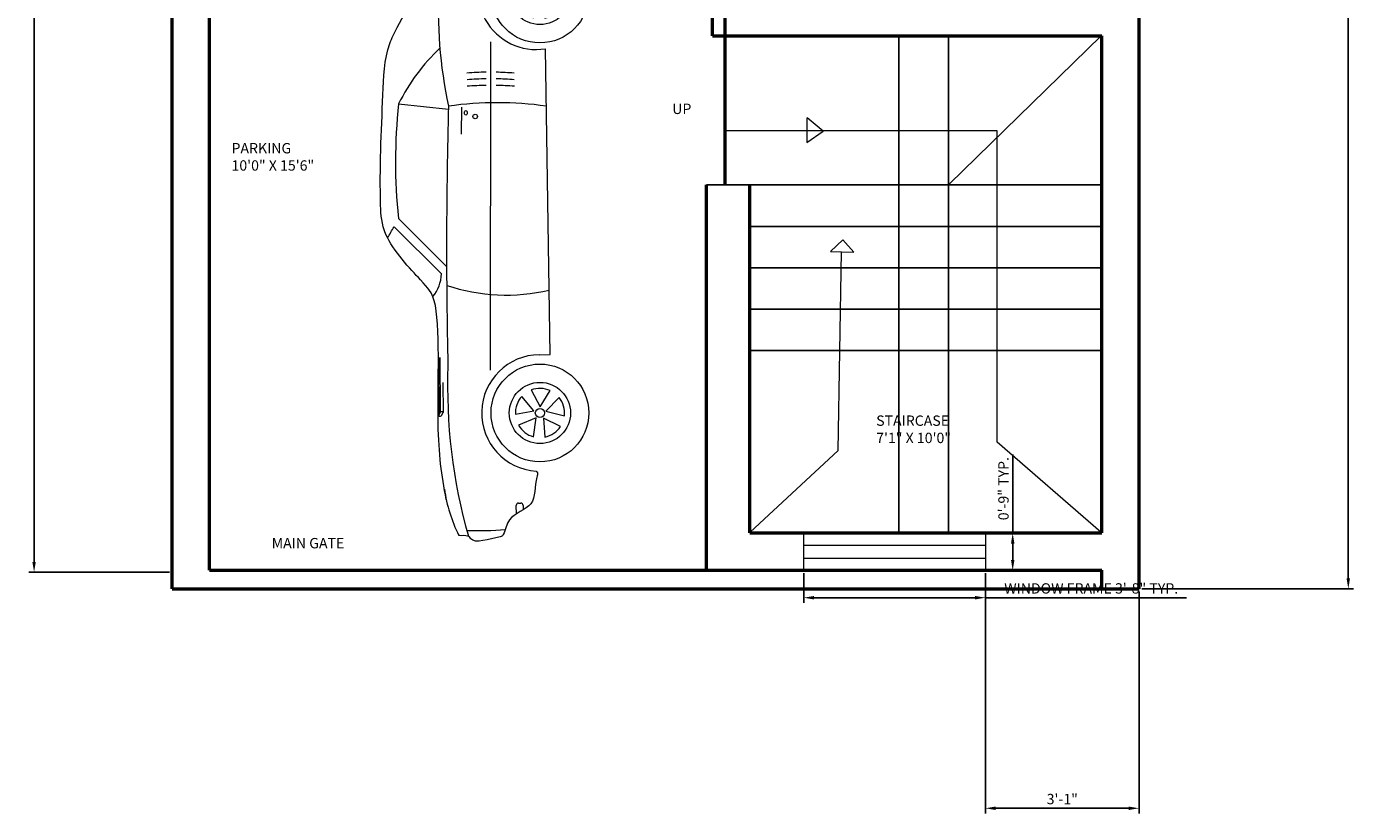
# Model space of a CAD drawing. Units: inches. Extents: x 210 to 950, y 0 to 561.
# Tile 1 of 5: x 228 to 548, y 0 to 190. Entities that reach past the tile are written whole.
import ezdxf

# ---------------------------------------------------------------- set-up
doc = ezdxf.new("R2010")
doc.units = ezdxf.units.IN
for name, color, linetype, lineweight in [('A-ANNO-DIMS', 2, 'Continuous', 18), ('A-ANNO-SYMB', 7, 'Continuous', 18), ('A-ANNO-TEXT', 7, 'Continuous', 18), ('A-AREA-IDEN', 7, 'Continuous', 18), ('A-FLOR-STRS', 7, 'Continuous', 25), ('A-GLAZ', 4, 'Continuous', 20), ('A-SITE-VEHI', 8, 'Continuous', 13), ('A-WALL', 7, 'Continuous', 50)]:
    doc.layers.add(name, color=color, linetype=linetype, lineweight=lineweight)
doc.styles.get("Standard").update_dxf_attribs({"font": 'arial.ttf'})
doc.dimstyles.new('ISO-25', dxfattribs={"dimtxt": 2.5, "dimasz": 2.5, "dimexe": 1.25, "dimexo": 0.625, "dimtad": 1, "dimtxsty": 'Standard', "dimcen": 2.5, "dimadec": 0, "dimazin": 0, "dimtfac": 1, "dimtmove": 0, "dimatfit": 3, "dimfxl": 1, "dimarcsym": 0})

# ---------------------------------------------------------------- blocks, each defined once
blk = doc.blocks.new('*U2')
for p, q in [((72.93, 40.23), (85.8, 53.18)), ((75, 38.82), (88.08, 51.97)), ((119.39, 51.91), (117.92, 38.32)), ((50.13, 41.06), (34.31, 40.98)), ((43.26, 39.85), (35.15, 39.78)), ((35.3, 40.46), (50.13, 40.62)), ((111.09, 34.73), (118.48, 34.64)), ((46.65, 26.83), (136.29, 26.77)), ((180.37, 26.17), (187.51, 26.41)), ((179.3, 24.35), (180.25, 22.49)), ((186.68, 22.17), (188.51, 24.37)), ((7.45, 19.78), (9.74, 19.8)), ((10.37, 19.19), (10.38, 18.56)), ((182.62, 21.14), (184.91, 21.28)), ((9.76, 17.93), (8.53, 17.92)), ((50.87, 13.52), (50.91, 10.52))]:
    blk.add_line(p, q)
for points in [[(35.31, 39.93), (35.3, 40.27, 0.269532), (35.14, 40.54), (34.38, 40.96, 0.575383), (34.15, 40.83), (34.15, 40.49, 0.269532), (34.32, 40.22), (35.08, 39.79, 0.575383)], [(28.49, 15.1), (33.61, 14.4), (31.65, 19.18, 0.199906)], [(34.64, 20.05), (35.56, 14.97), (39.5, 18.31, 0.199906)], [(142.85, 15.1), (147.96, 14.4), (146.01, 19.18, 0.199906)], [(148.99, 20.05), (149.91, 14.97), (153.85, 18.31, 0.199906)], [(41.25, 15.74), (36.7, 13.3), (41.09, 10.58, 0.199906)], [(155.6, 15.74), (151.06, 13.3), (155.45, 10.58, 0.199906)], [(31.31, 7.72), (33.55, 12.37), (28.4, 11.99, 0.199906)], [(39.19, 8.12), (35.46, 11.69), (34.23, 6.67, 0.199906)], [(145.66, 7.72), (147.9, 12.37), (142.75, 11.99, 0.199906)], [(153.54, 8.12), (149.81, 11.69), (148.59, 6.67, 0.199906)]]:
    blk.add_lwpolyline(points, format="xyb", close=True)
for points in [[(181.58, 27.46), (181.53, 31.95), (180.48, 32.43)], [(181.58, 27.46), (181.53, 31.95), (182.57, 32.45)], [(50.91, 10.52), (134.38, 11.83)]]:
    blk.add_lwpolyline(points)
for centre, radius in [((115.89, 31.01), 0.619), ((34.98, 13.35), 13.35), ((149.33, 13.35), 13.35), ((34.98, 13.35), 8.35), ((149.33, 13.35), 8.35), ((34.98, 13.35), 1.25), ((149.33, 13.35), 1.25)]:
    blk.add_circle(centre, radius)
for centre, radius, start, end in [((114.6, 105.09), 59.37, 237.6103, 240.9785), ((103.45, -95), 147.78, 83.8163, 95.9705), ((95.51, 3.91), 53.61, 43.2748, 63.5665), ((73.29, 50.49), 10.26, 230.424, 268.0085), ((145.17, -84.88), 125.99, 71.5283, 102.1242), ((42.18, -111.35), 149.91, 87.8393, 105.8096), ((20.53, -3.15), 43.06, 98.5304, 116.112), ((80.1, -1364.13), 1402.96, 88.42296, 91.3179), ((118.31, 22.51), 51.16, 161.4307, 193.2363), ((25.66, 24.94), 94.01, 351.8279, 8.1674), ((79.16, 30.11), 76.3, 177.5773, 185.5205), ((45.64, 26.83), 78.76, 0.852, 4.6556), ((47.43, 26.85), 78.76, 0.852, 4.6556), ((49.23, 26.87), 78.76, 0.852, 4.6556), ((184.3, 32.25), 2.49, 357.932, 71.5283), ((34.98, 13.35), 15.9, 0.6373, 176.3412), ((150.1, 14.36), 15.92, 49.2263, 189.1528), ((216.26, 37.76), 36.17, 188.4683, 196.5315), ((146.68, 36.98), 36.17, 344.7432, 352.8063), ((116.55, 34.7), 70.29, 353.1942, 357.932), ((149.4, 16.55), 14.84, 352.7285, 41.6613), ((180.41, 24.92), 1.25, 91.939, 207.109), ((187.55, 25.16), 1.25, 320.1683, 91.939), ((45.64, 26.83), 78.76, 355.2644, 358.8633), ((47.43, 26.85), 78.76, 355.2644, 358.8633), ((49.23, 26.87), 78.76, 355.2644, 358.8633), ((182.47, 23.63), 2.49, 207.109, 273.4677), ((184.76, 23.76), 2.49, 273.4677, 320.1683), ((9.75, 19.18), 0.623, 0.6373, 90.6373), ((9.76, 18.55), 0.623, 270.6373, 0.6373), ((162.47, 70.82), 56.18, 271.6865, 290.2774), ((114.25, 37.03), 70.29, 344.3985, 346.9385)]:
    blk.add_arc(centre, radius, start, end)
blk.add_ellipse((116.89, 33.59), major_axis=(-0.63, -0.007), ratio=0.610043)
for points, knots in [([(11.39, 38.92), (18.06, 40.19), (30.91, 42.01), (64.77, 40.11), (70.25, 44.91), (82.35, 56.38), (99.18, 57.3), (116.06, 56.35), (133.04, 55.87), (145.24, 49.87), (153.62, 43.8), (161.17, 40.68), (164.92, 39.73), (167.29, 39.15)], [18.629823, 18.629823, 18.629823, 18.629823, 19.527405, 20.700571, 21.107983, 21.608568, 21.92336, 23.151359, 23.716171, 23.908743, 24.77794, 24.943072, 25.187755, 25.187755, 25.187755, 25.187755]), ([(19.11, 14.36), (18.99, 14.21), (18.5, 13.81), (15.35, 15), (9.19, 13.94), (7.26, 22.22), (3.01, 22.66), (1.32, 23.61), (0.64, 26.92), (-0.96, 31.49), (1.54, 32.64), (1.5, 34.06), (1.49, 34.8), (1.49, 35.06), (1.52, 35.3), (1.58, 35.51)], [16.815853, 16.815853, 16.815853, 16.815853, 16.838212, 16.885395, 17.18439, 17.479846, 17.654423, 17.670693, 17.696923, 18.016358, 18.052739, 18.140805, 18.140805, 18.140805, 18.172382, 18.172382, 18.172382, 18.172382])]:
    blk.add_open_spline(points, degree=3, knots=knots)
blk = doc.blocks.new('*D15')
at = {"layer": 'A-ANNO-DIMS', "color": 0, "lineweight": -2, "transparency": 16777216}
for p, q in [((262.29, 538.5), (228.3, 538.5)), ((229.55, 61), (229.55, 536)), ((262.29, 58.5), (228.3, 58.5))]:
    blk.add_line(p, q, dxfattribs=at)
at = {"layer": 'A-ANNO-DIMS', "color": 0, "transparency": 16777216}
for points in [[(229.13, 536), (229.96, 536), (229.55, 538.5)], [(229.13, 61), (229.96, 61), (229.55, 58.5)]]:
    blk.add_solid(points, dxfattribs=at)
at = {"layer": 'Defpoints', "color": 0, "transparency": 16777216}
for p in [(229.55, 538.5), (262.91, 538.5), (262.91, 58.5)]:
    blk.add_point(p, dxfattribs=at)
at = {"layer": 'A-ANNO-DIMS', "color": 0, "transparency": 16777216, "insert": (228.41, 298.5), "char_height": 1, "attachment_point": 5, "rotation": 90}
blk.add_mtext("40'", dxfattribs=at)
blk = doc.blocks.new('*D16')
at = {"layer": 'A-ANNO-DIMS', "color": 0, "lineweight": -2, "transparency": 16777216}
for p, q in [((497.04, 538.5), (548.19, 538.5)), ((546.94, 57), (546.94, 536)), ((497.04, 54.5), (548.19, 54.5))]:
    blk.add_line(p, q, dxfattribs=at)
at = {"layer": 'A-ANNO-DIMS', "color": 0, "transparency": 16777216}
for points in [[(546.52, 536), (547.35, 536), (546.94, 538.5)], [(546.52, 57), (547.35, 57), (546.94, 54.5)]]:
    blk.add_solid(points, dxfattribs=at)
at = {"layer": 'Defpoints', "color": 0, "transparency": 16777216}
for p in [(496.41, 538.5), (546.94, 538.5), (496.41, 54.5)]:
    blk.add_point(p, dxfattribs=at)
at = {"layer": 'A-ANNO-DIMS', "color": 0, "transparency": 16777216, "insert": (545.8, 296.5), "char_height": 1, "attachment_point": 5, "rotation": 90}
blk.add_mtext('40\'-4"', dxfattribs=at)
blk = doc.blocks.new('WIN-44IN-DEEP-FRAME')
for p, q in [((0, 0), (0, 9)), ((0, 9), (43.89, 9)), ((43.89, 9), (43.89, 0)), ((43.89, 6), (0, 6)), ((0, 3), (43.89, 3)), ((43.89, 0), (0, 0))]:
    blk.add_line(p, q)
blk = doc.blocks.new('*D24')
at = {"layer": 'A-ANNO-DIMS', "color": 0, "lineweight": -2, "transparency": 16777216}
for p, q in [((415.41, 58.31), (415.41, 51.1)), ((459.31, 58.31), (459.31, 51.1)), ((417.91, 52.35), (456.81, 52.35)), ((459.31, 52.35), (507.89, 52.35))]:
    blk.add_line(p, q, dxfattribs=at)
at = {"layer": 'A-ANNO-DIMS', "color": 0, "transparency": 16777216}
for points in [[(417.91, 52.77), (417.91, 51.93), (415.41, 52.35)], [(456.81, 52.77), (456.81, 51.93), (459.31, 52.35)]]:
    blk.add_solid(points, dxfattribs=at)
at = {"layer": 'Defpoints', "color": 0, "transparency": 16777216}
for p in [(415.41, 58.93), (459.31, 58.93), (459.31, 52.35)]:
    blk.add_point(p, dxfattribs=at)
at = {"layer": 'A-ANNO-DIMS', "color": 0, "transparency": 16777216, "insert": (484.85, 54.27), "char_height": 2.5, "attachment_point": 5}
blk.add_mtext('WINDOW FRAME 3\'-8" TYP.', dxfattribs=at)
blk = doc.blocks.new('*D25')
at = {"layer": 'A-ANNO-DIMS', "color": 0, "lineweight": -2, "transparency": 16777216}
for p, q in [((465.89, 67.93), (465.89, 86.92)), ((459.93, 67.93), (467.14, 67.93)), ((465.89, 61.43), (465.89, 65.43)), ((459.93, 58.93), (467.14, 58.93))]:
    blk.add_line(p, q, dxfattribs=at)
at = {"layer": 'A-ANNO-DIMS', "color": 0, "transparency": 16777216}
for points in [[(465.48, 65.43), (466.31, 65.43), (465.89, 67.93)], [(465.48, 61.43), (466.31, 61.43), (465.89, 58.93)]]:
    blk.add_solid(points, dxfattribs=at)
at = {"layer": 'Defpoints', "color": 0, "transparency": 16777216}
for p in [(459.31, 67.93), (465.89, 67.93), (459.31, 58.93)]:
    blk.add_point(p, dxfattribs=at)
at = {"layer": 'A-ANNO-DIMS', "color": 0, "transparency": 16777216, "insert": (463.99, 78.68), "char_height": 2.5, "attachment_point": 5, "rotation": 90}
blk.add_mtext('0\'-9" TYP.', dxfattribs=at)
blk = doc.blocks.new('*D49')
at = {"layer": 'A-ANNO-DIMS', "color": 0, "lineweight": -2, "transparency": 16777216}
for p, q in [((459.31, 58.31), (459.31, 0.26)), ((496.41, 53.88), (496.41, 0.26)), ((461.81, 1.51), (493.91, 1.51))]:
    blk.add_line(p, q, dxfattribs=at)
at = {"layer": 'A-ANNO-DIMS', "color": 0, "transparency": 16777216}
for points in [[(461.81, 1.93), (461.81, 1.09), (459.31, 1.51)], [(493.91, 1.93), (493.91, 1.09), (496.41, 1.51)]]:
    blk.add_solid(points, dxfattribs=at)
at = {"layer": 'Defpoints', "color": 0, "transparency": 16777216}
for p in [(459.31, 58.93), (496.41, 54.5), (496.41, 1.51)]:
    blk.add_point(p, dxfattribs=at)
at = {"layer": 'A-ANNO-DIMS', "color": 0, "transparency": 16777216, "insert": (477.86, 3.41), "char_height": 2.5, "attachment_point": 5}
blk.add_mtext('3\'-1"', dxfattribs=at)

msp = doc.modelspace()

# ---------------------------------------------------------------- linework, layer by layer
at = {"layer": 'A-ANNO-SYMB'}
for p, q in [((416.2, 168.24), (416.2, 162.26)), ((420.12, 164.96), (416.25, 168.24)), ((462.15, 165.07), (396.41, 165.07)), ((416.2, 162.26), (420.12, 164.96)), ((462.15, 89.9), (462.15, 165.07)), ((424.88, 138.72), (421.85, 135.94)), ((427.54, 135.79), (424.88, 138.72)), ((421.85, 135.94), (424.58, 135.88)), ((423.74, 87.93), (424.54, 135.89)), ((424.54, 135.89), (427.54, 135.79)), ((487.17, 68.15), (462.15, 89.9)), ((402.5, 68.18), (423.74, 87.93))]:
    msp.add_line(p, q, dxfattribs=at)
at = {"layer": 'A-FLOR-STRS'}
for p, q in [((438.41, 68), (438.41, 188)), ((450.41, 68), (450.41, 188)), ((450.51, 152.23), (487.29, 187.98)), ((391.91, 152), (487.41, 152)), ((402.41, 142), (487.41, 142)), ((402.41, 132), (487.41, 132)), ((402.41, 122), (487.41, 122)), ((402.41, 112), (487.41, 112))]:
    msp.add_line(p, q, dxfattribs=at)
at = {"layer": 'A-WALL'}
for p, q in [((262.91, 54.5), (262.91, 538.5)), ((496.41, 54.5), (496.41, 538.5)), ((393.41, 188), (393.41, 249.5)), ((396.41, 152), (396.41, 249.5)), ((271.91, 59), (271.91, 240.5)), ((393.41, 188), (487.41, 188)), ((487.41, 68), (487.41, 188)), ((391.91, 59), (391.91, 152)), ((402.41, 68), (402.41, 152)), ((402.41, 68), (487.41, 68)), ((271.91, 59), (391.91, 59)), ((391.91, 59), (487.41, 59)), ((487.41, 54.5), (487.41, 59)), ((262.91, 54.5), (496.41, 54.5))]:
    msp.add_line(p, q, dxfattribs=at)

# ---------------------------------------------------------------- block references
at = {"layer": 'A-GLAZ'}
msp.add_blockref('WIN-44IN-DEEP-FRAME', (415.41, 58.93), dxfattribs=at)
at = {"layer": 'A-SITE-VEHI', "xscale": 0.8846285948067201, "yscale": 0.8846285948067201, "zscale": 0.8846285948067201, "rotation": 90}
msp.add_blockref('*U2', (363.52, 66.01), dxfattribs=at)

# ---------------------------------------------------------------- texts
at = {"layer": 'A-ANNO-TEXT', "char_height": 2.5, "attachment_point": 1}
for s, width, insert in [('UP ', 6.3402, (383.67, 171.63)), ('MAIN GATE', 20.3678, (286.93, 66.77))]:
    msp.add_mtext_dynamic_manual_height_columns(s, width=width, gutter_width=12.5, heights=[0], dxfattribs=dict(at, insert=insert))
at = {"layer": 'A-AREA-IDEN', "char_height": 2.5, "attachment_point": 1}
for s, width, insert in [('PARKING\\P10\'0" X 15\'6"', 25.7748, (277.23, 162.13)), ('STAIRCASE\\P\\pxt4;7\'1" X 10\'0"', 29.1994, (432.92, 96.35))]:
    msp.add_mtext_dynamic_manual_height_columns(s, width=width, gutter_width=12.5, heights=[0], dxfattribs=dict(at, insert=insert))

# ---------------------------------------------------------------- dimensions: what is measured, and where the dimension line sits
at = {"layer": 'A-ANNO-DIMS'}
for base, p1, p2, picture, middle in [((229.55, 538.5), (262.91, 58.5), (262.91, 538.5), '*D15', (228.41, 298.5)), ((546.94, 538.5), (496.41, 54.5), (496.41, 538.5), '*D16', (545.8, 296.5))]:
    dim = msp.add_linear_dim(base=base, p1=p1, p2=p2, angle=90, dimstyle='ISO-25', override={"dimtxt": 1, "dimdec": 0, "dimlunit": 3, "dimclrd": 0, "dimclre": 0, "dimclrt": 0, "dimtdec": 0}, dxfattribs=at)
    dim.commit()
    dim.dimension.update_dxf_attribs({"geometry": picture, "text_midpoint": middle})
dim = msp.add_linear_dim(base=(465.89, 67.93), p1=(459.31, 58.93), p2=(459.31, 67.93), angle=90, text='<> TYP.', dimstyle='ISO-25', override={"dimdec": 1, "dimlfac": 1, "dimrnd": 0, "dimzin": 1, "dimdsep": 46, "dimlunit": 4, "dimfrac": 2}, dxfattribs=at)
dim.commit()
dim.dimension.update_dxf_attribs({"geometry": '*D25', "text_midpoint": (463.99, 78.68)})
dim = msp.add_linear_dim(base=(459.31, 52.35), p1=(415.41, 58.93), p2=(459.31, 58.93), text='WINDOW FRAME <> TYP.', dimstyle='ISO-25', override={"dimdec": 1, "dimlfac": 1, "dimrnd": 0, "dimzin": 1, "dimdsep": 46, "dimlunit": 4, "dimfrac": 2}, dxfattribs=at)
dim.commit()
dim.dimension.update_dxf_attribs({"geometry": '*D24', "text_midpoint": (484.85, 54.27)})
dim = msp.add_linear_dim(base=(496.41, 1.51), p1=(459.31, 58.93), p2=(496.41, 54.5), dimstyle='ISO-25', override={"dimdec": 1, "dimlfac": 1, "dimrnd": 0, "dimzin": 1, "dimdsep": 46, "dimlunit": 4, "dimfrac": 2}, dxfattribs=at)
dim.commit()
dim.dimension.update_dxf_attribs({"geometry": '*D49', "text_midpoint": (477.86, 3.41)})

doc.saveas('drawing.dxf')
